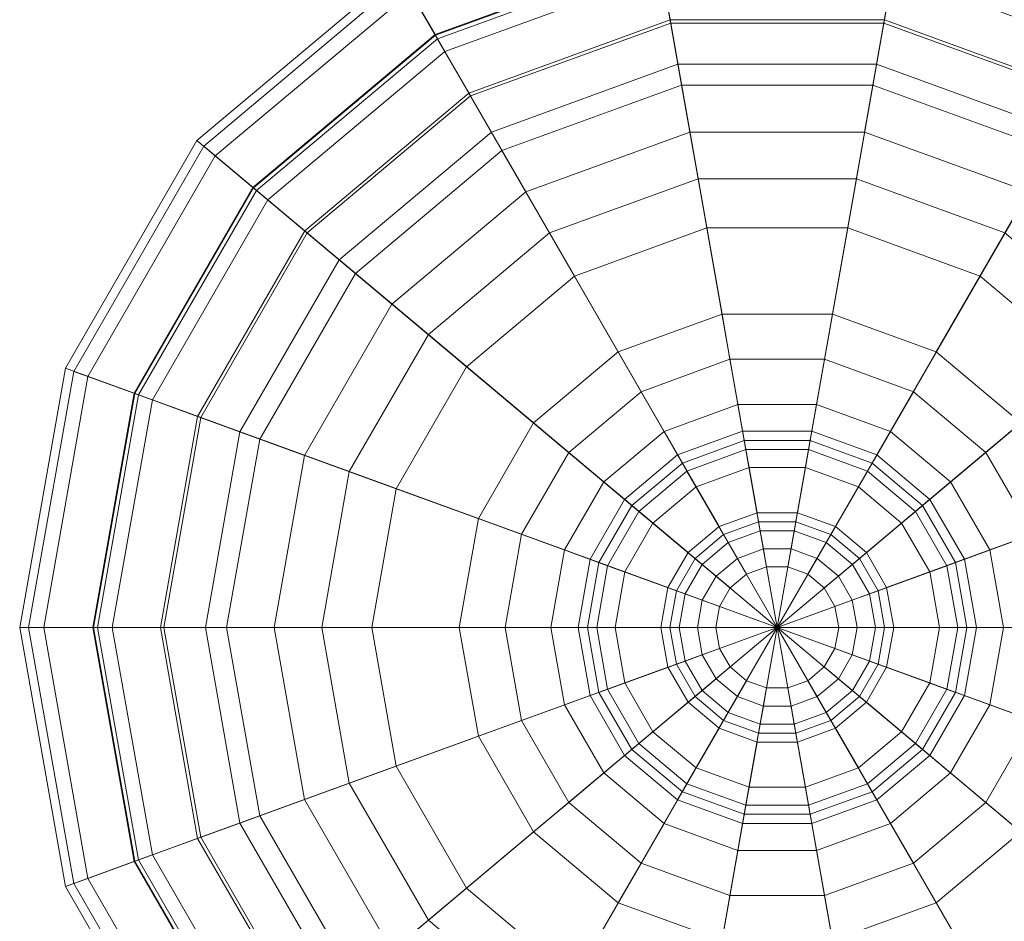
# Model space of a CAD drawing. Units: inches. Extents: x 375 to 1122, y 27 to 1069.
# Tile 120 of 155: x 717.909 to 719.669, y 890.59 to 892.201. Entities that reach past the tile are written whole.
import ezdxf

# ---------------------------------------------------------------- set-up
doc = ezdxf.new("R2010")
doc.units = ezdxf.units.IN
doc.layers.add('Furniture', color=30, linetype='Continuous', lineweight=18)

# ---------------------------------------------------------------- blocks, each defined once
blk = doc.blocks.new('A$C403C54AD')
for points in [[(1.180252, 0.891746, -0.031825), (1.180252, 0.857884, -0.028747), (1.180252, 0.857884, -0.028747), (1.16867, 0.889704, -0.031825)], [(1.191834, 0.889704, -0.031825), (1.180252, 0.857884, -0.028747), (1.180252, 0.857884, -0.028747), (1.180252, 0.891746, -0.031825)], [(1.16867, 0.889704, -0.031825), (1.180252, 0.857884, -0.028747), (1.180252, 0.857884, -0.028747), (1.158486, 0.883824, -0.031825)], [(1.202018, 0.883824, -0.031825), (1.180252, 0.857884, -0.028747), (1.180252, 0.857884, -0.028747), (1.191834, 0.889704, -0.031825)], [(1.158486, 0.883824, -0.031825), (1.180252, 0.857884, -0.028747), (1.180252, 0.857884, -0.028747), (1.150927, 0.874815, -0.031825)], [(1.209578, 0.874815, -0.031825), (1.180252, 0.857884, -0.028747), (1.180252, 0.857884, -0.028747), (1.202018, 0.883824, -0.031825)], [(1.171115, 0.868773, -0.02532), (1.160585, 0.881322, -0.028594), (1.153755, 0.873182, -0.028594), (1.167942, 0.864991, -0.02532)], [(1.192562, 0.864991, -0.02532), (1.206749, 0.873182, -0.028594), (1.199919, 0.881322, -0.028594), (1.189389, 0.868773, -0.02532)], [(1.180252, 0.878242, 0.061451), (1.180252, 0.868003, 0.054084), (1.176791, 0.867392, 0.054084), (1.173289, 0.877014, 0.061451)], [(1.187215, 0.877014, 0.061451), (1.183713, 0.867392, 0.054084), (1.180252, 0.868003, 0.054084), (1.180252, 0.878242, 0.061451)], [(1.1686, 0.87177, 0.063639), (1.164431, 0.876739, 0.073031), (1.158936, 0.87019, 0.073031), (1.164553, 0.866948, 0.063639)], [(1.173289, 0.877014, 0.061451), (1.176791, 0.867392, 0.054084), (1.173748, 0.865635, 0.054084), (1.167166, 0.873479, 0.061451)], [(1.193338, 0.873479, 0.061451), (1.186756, 0.865635, 0.054084), (1.183713, 0.867392, 0.054084), (1.187215, 0.877014, 0.061451)], [(1.195951, 0.866948, 0.063639), (1.201568, 0.87019, 0.073031), (1.196073, 0.876739, 0.073031), (1.191904, 0.87177, 0.063639)], [(1.180252, 0.866788, 0.057003), (1.180252, 0.876011, 0.063639), (1.174052, 0.874918, 0.063639), (1.177207, 0.866251, 0.057003)], [(1.183297, 0.866251, 0.057003), (1.186452, 0.874918, 0.063639), (1.180252, 0.876011, 0.063639), (1.180252, 0.866788, 0.057003)], [(1.153755, 0.873182, -0.028594), (1.150927, 0.874815, -0.031825), (1.146904, 0.863764, -0.031825), (1.15012, 0.863197, -0.028594)], [(1.150927, 0.874815, -0.031825), (1.180252, 0.857884, -0.028747), (1.180252, 0.857884, -0.028747), (1.146904, 0.863764, -0.031825)], [(1.15379, 0.873162, 0.131159), (1.151272, 0.874616, 0.117935), (1.147297, 0.863695, 0.117935), (1.15016, 0.86319, 0.131159)], [(1.177207, 0.866251, 0.057003), (1.174052, 0.874918, 0.063639), (1.1686, 0.87177, 0.063639), (1.174529, 0.864705, 0.057003)], [(1.2136, 0.863764, -0.031825), (1.180252, 0.857884, -0.028747), (1.180252, 0.857884, -0.028747), (1.209578, 0.874815, -0.031825)], [(1.185975, 0.864705, 0.057003), (1.191904, 0.87177, 0.063639), (1.186452, 0.874918, 0.063639), (1.183297, 0.866251, 0.057003)], [(1.151856, 0.874278, 0.089693), (1.156502, 0.871596, 0.071684), (1.153245, 0.862646, 0.071684), (1.147962, 0.863578, 0.089693)], [(1.167942, 0.864991, -0.02532), (1.153755, 0.873182, -0.028594), (1.15012, 0.863197, -0.028594), (1.166254, 0.860352, -0.02532)], [(1.167166, 0.873479, 0.061451), (1.173748, 0.865635, 0.054084), (1.171489, 0.862943, 0.054084), (1.162622, 0.868063, 0.061451)], [(1.197882, 0.868063, 0.061451), (1.189015, 0.862943, 0.054084), (1.186756, 0.865635, 0.054084), (1.193338, 0.873479, 0.061451)], [(1.19425, 0.860352, -0.02532), (1.210384, 0.863197, -0.028594), (1.206749, 0.873182, -0.028594), (1.192562, 0.864991, -0.02532)], [(1.158117, 0.870664, 0.140564), (1.15379, 0.873162, 0.131159), (1.15016, 0.86319, 0.131159), (1.155081, 0.862322, 0.140564)], [(1.153943, 0.873073, 0.117718), (1.156376, 0.871669, 0.130354), (1.153102, 0.862671, 0.130354), (1.150335, 0.863159, 0.117718)], [(1.154513, 0.872744, 0.090178), (1.153943, 0.873073, 0.117718), (1.150335, 0.863159, 0.117718), (1.150983, 0.863045, 0.090178)], [(1.158936, 0.87019, 0.073031), (1.154513, 0.872744, 0.090178), (1.150983, 0.863045, 0.090178), (1.156013, 0.862158, 0.073031)], [(1.156376, 0.871669, 0.130354), (1.160783, 0.869125, 0.140564), (1.158112, 0.861788, 0.140564), (1.153102, 0.862671, 0.130354)], [(1.156502, 0.871596, 0.071684), (1.162622, 0.868063, 0.061451), (1.160204, 0.861419, 0.061451), (1.153245, 0.862646, 0.071684)], [(1.174529, 0.864705, 0.057003), (1.1686, 0.87177, 0.063639), (1.164553, 0.866948, 0.063639), (1.172541, 0.862336, 0.057003)], [(1.187963, 0.862336, 0.057003), (1.195951, 0.866948, 0.063639), (1.191904, 0.87177, 0.063639), (1.185975, 0.864705, 0.057003)], [(1.176091, 0.869317, -0.022455), (1.17539, 0.871241, -0.02532), (1.171115, 0.868773, -0.02532), (1.172432, 0.867204, -0.022455)], [(1.188073, 0.867204, -0.022455), (1.189389, 0.868773, -0.02532), (1.185114, 0.871241, -0.02532), (1.184413, 0.869317, -0.022455)], [(1.160783, 0.869125, 0.140564), (1.158117, 0.870664, 0.140564), (1.155081, 0.862322, 0.140564), (1.158112, 0.861788, 0.140564)], [(1.164553, 0.866948, 0.063639), (1.158936, 0.87019, 0.073031), (1.156013, 0.862158, 0.073031), (1.1624, 0.861032, 0.063639)], [(1.180252, 0.865955, -0.020408), (1.180252, 0.87005, -0.022455), (1.176091, 0.869317, -0.022455), (1.177492, 0.865468, -0.020408)], [(1.183012, 0.865468, -0.020408), (1.184413, 0.869317, -0.022455), (1.180252, 0.87005, -0.022455), (1.180252, 0.865955, -0.020408)], [(1.177492, 0.865468, -0.020408), (1.176091, 0.869317, -0.022455), (1.172432, 0.867204, -0.022455), (1.175064, 0.864067, -0.020408)], [(1.18544, 0.864067, -0.020408), (1.188073, 0.867204, -0.022455), (1.184413, 0.869317, -0.022455), (1.183012, 0.865468, -0.020408)], [(1.172432, 0.867204, -0.022455), (1.171115, 0.868773, -0.02532), (1.167942, 0.864991, -0.02532), (1.169716, 0.863967, -0.022455)], [(1.190789, 0.863967, -0.022455), (1.192562, 0.864991, -0.02532), (1.189389, 0.868773, -0.02532), (1.188073, 0.867204, -0.022455)], [(1.162622, 0.868063, 0.061451), (1.171489, 0.862943, 0.054084), (1.170287, 0.859641, 0.054084), (1.160204, 0.861419, 0.061451)], [(1.180252, 0.868003, 0.054084), (1.180252, 0.863088, 0.053266), (1.178472, 0.862774, 0.053266), (1.176791, 0.867392, 0.054084)], [(1.183713, 0.867392, 0.054084), (1.182032, 0.862774, 0.053266), (1.180252, 0.863088, 0.053266), (1.180252, 0.868003, 0.054084)], [(1.2003, 0.861419, 0.061451), (1.190217, 0.859641, 0.054084), (1.189015, 0.862943, 0.054084), (1.197882, 0.868063, 0.061451)], [(1.175064, 0.864067, -0.020408), (1.172432, 0.867204, -0.022455), (1.169716, 0.863967, -0.022455), (1.173262, 0.861919, -0.020408)], [(1.176791, 0.867392, 0.054084), (1.178472, 0.862774, 0.053266), (1.176907, 0.861871, 0.053266), (1.173748, 0.865635, 0.054084)], [(1.186756, 0.865635, 0.054084), (1.183597, 0.861871, 0.053266), (1.182032, 0.862774, 0.053266), (1.183713, 0.867392, 0.054084)], [(1.187242, 0.861919, -0.020408), (1.190789, 0.863967, -0.022455), (1.188073, 0.867204, -0.022455), (1.18544, 0.864067, -0.020408)], [(1.172541, 0.862336, 0.057003), (1.164553, 0.866948, 0.063639), (1.1624, 0.861032, 0.063639), (1.171483, 0.85943, 0.057003)], [(1.180252, 0.857884, 0.055519), (1.180252, 0.866788, 0.057003), (1.177207, 0.866251, 0.057003), (1.180252, 0.857884, 0.055519)], [(1.180252, 0.857884, 0.055519), (1.183297, 0.866251, 0.057003), (1.180252, 0.866788, 0.057003), (1.180252, 0.857884, 0.055519)], [(1.189021, 0.85943, 0.057003), (1.198104, 0.861032, 0.063639), (1.195951, 0.866948, 0.063639), (1.187963, 0.862336, 0.057003)], [(1.180252, 0.857884, 0.055519), (1.177207, 0.866251, 0.057003), (1.174529, 0.864705, 0.057003), (1.180252, 0.857884, 0.055519)], [(1.180252, 0.866365, 0.0504), (1.180252, 0.862269, 0.048354), (1.178752, 0.862005, 0.048354), (1.177352, 0.865853, 0.0504)], [(1.180252, 0.865136, 0.052447), (1.180252, 0.866365, 0.0504), (1.177352, 0.865853, 0.0504), (1.177772, 0.864699, 0.052447)], [(1.183153, 0.865853, 0.0504), (1.181752, 0.862005, 0.048354), (1.180252, 0.862269, 0.048354), (1.180252, 0.866365, 0.0504)], [(1.182732, 0.864699, 0.052447), (1.183153, 0.865853, 0.0504), (1.180252, 0.866365, 0.0504), (1.180252, 0.865136, 0.052447)], [(1.180252, 0.857884, 0.055519), (1.185975, 0.864705, 0.057003), (1.183297, 0.866251, 0.057003), (1.180252, 0.857884, 0.055519)], [(1.177352, 0.865853, 0.0504), (1.178752, 0.862005, 0.048354), (1.177433, 0.861243, 0.048354), (1.174801, 0.86438, 0.0504)], [(1.177772, 0.864699, 0.052447), (1.177352, 0.865853, 0.0504), (1.174801, 0.86438, 0.0504), (1.175591, 0.863439, 0.052447)], [(1.180252, 0.862679, -0.015087), (1.180252, 0.865955, -0.020408), (1.177492, 0.865468, -0.020408), (1.178612, 0.862389, -0.015087)], [(1.181892, 0.862389, -0.015087), (1.183012, 0.865468, -0.020408), (1.180252, 0.865955, -0.020408), (1.180252, 0.862679, -0.015087)], [(1.185703, 0.86438, 0.0504), (1.183071, 0.861243, 0.048354), (1.181752, 0.862005, 0.048354), (1.183153, 0.865853, 0.0504)], [(1.184913, 0.863439, 0.052447), (1.185703, 0.86438, 0.0504), (1.183153, 0.865853, 0.0504), (1.182732, 0.864699, 0.052447)], [(1.173748, 0.865635, 0.054084), (1.176907, 0.861871, 0.053266), (1.175745, 0.860486, 0.053266), (1.171489, 0.862943, 0.054084)], [(1.178612, 0.862389, -0.015087), (1.177492, 0.865468, -0.020408), (1.175064, 0.864067, -0.020408), (1.17717, 0.861557, -0.015087)], [(1.183334, 0.861557, -0.015087), (1.18544, 0.864067, -0.020408), (1.183012, 0.865468, -0.020408), (1.181892, 0.862389, -0.015087)], [(1.189015, 0.862943, 0.054084), (1.184759, 0.860486, 0.053266), (1.183597, 0.861871, 0.053266), (1.186756, 0.865635, 0.054084)], [(1.169716, 0.863967, -0.022455), (1.167942, 0.864991, -0.02532), (1.166254, 0.860352, -0.02532), (1.16827, 0.859997, -0.022455)], [(1.180252, 0.863088, 0.053266), (1.180252, 0.865136, 0.052447), (1.177772, 0.864699, 0.052447), (1.178472, 0.862774, 0.053266)], [(1.182032, 0.862774, 0.053266), (1.182732, 0.864699, 0.052447), (1.180252, 0.865136, 0.052447), (1.180252, 0.863088, 0.053266)], [(1.192234, 0.859997, -0.022455), (1.19425, 0.860352, -0.02532), (1.192562, 0.864991, -0.02532), (1.190789, 0.863967, -0.022455)], [(1.180252, 0.857884, 0.055519), (1.174529, 0.864705, 0.057003), (1.172541, 0.862336, 0.057003), (1.180252, 0.857884, 0.055519)], [(1.174801, 0.86438, 0.0504), (1.177433, 0.861243, 0.048354), (1.176454, 0.860076, 0.048354), (1.172908, 0.862124, 0.0504)], [(1.175591, 0.863439, 0.052447), (1.174801, 0.86438, 0.0504), (1.172908, 0.862124, 0.0504), (1.173972, 0.86151, 0.052447)], [(1.178472, 0.862774, 0.053266), (1.177772, 0.864699, 0.052447), (1.175591, 0.863439, 0.052447), (1.176907, 0.861871, 0.053266)], [(1.180252, 0.857884, 0.055519), (1.187963, 0.862336, 0.057003), (1.185975, 0.864705, 0.057003), (1.180252, 0.857884, 0.055519)], [(1.183597, 0.861871, 0.053266), (1.184913, 0.863439, 0.052447), (1.182732, 0.864699, 0.052447), (1.182032, 0.862774, 0.053266)], [(1.187596, 0.862124, 0.0504), (1.18405, 0.860076, 0.048354), (1.183071, 0.861243, 0.048354), (1.185703, 0.86438, 0.0504)], [(1.186532, 0.86151, 0.052447), (1.187596, 0.862124, 0.0504), (1.185703, 0.86438, 0.0504), (1.184913, 0.863439, 0.052447)], [(1.173262, 0.861919, -0.020408), (1.169716, 0.863967, -0.022455), (1.16827, 0.859997, -0.022455), (1.172304, 0.859285, -0.020408)], [(1.17717, 0.861557, -0.015087), (1.175064, 0.864067, -0.020408), (1.173262, 0.861919, -0.020408), (1.1761, 0.860281, -0.015087)], [(1.184404, 0.860281, -0.015087), (1.187242, 0.861919, -0.020408), (1.18544, 0.864067, -0.020408), (1.183334, 0.861557, -0.015087)], [(1.1882, 0.859285, -0.020408), (1.192234, 0.859997, -0.022455), (1.190789, 0.863967, -0.022455), (1.187242, 0.861919, -0.020408)], [(1.146904, 0.863764, -0.031825), (1.180252, 0.857884, -0.028747), (1.180252, 0.857884, -0.028747), (1.146904, 0.852004, -0.031825)], [(1.147962, 0.863578, 0.089693), (1.153245, 0.862646, 0.071684), (1.153245, 0.853122, 0.071684), (1.147962, 0.85219, 0.089693)], [(1.2136, 0.852004, -0.031825), (1.180252, 0.857884, -0.028747), (1.180252, 0.857884, -0.028747), (1.2136, 0.863764, -0.031825)], [(1.166254, 0.860352, -0.02532), (1.15012, 0.863197, -0.028594), (1.15012, 0.852571, -0.028594), (1.166254, 0.855416, -0.02532)], [(1.155081, 0.862322, 0.140564), (1.15016, 0.86319, 0.131159), (1.15016, 0.852578, 0.131159), (1.155081, 0.853446, 0.140564)], [(1.150335, 0.863159, 0.117718), (1.153102, 0.862671, 0.130354), (1.153102, 0.853097, 0.130354), (1.150335, 0.852609, 0.117718)], [(1.176907, 0.861871, 0.053266), (1.175591, 0.863439, 0.052447), (1.173972, 0.86151, 0.052447), (1.175745, 0.860486, 0.053266)], [(1.184759, 0.860486, 0.053266), (1.186532, 0.86151, 0.052447), (1.184913, 0.863439, 0.052447), (1.183597, 0.861871, 0.053266)], [(1.156013, 0.862158, 0.073031), (1.150983, 0.863045, 0.090178), (1.150983, 0.852723, 0.090178), (1.156013, 0.85361, 0.073031)], [(1.153102, 0.862671, 0.130354), (1.158112, 0.861788, 0.140564), (1.158112, 0.85398, 0.140564), (1.153102, 0.853097, 0.130354)], [(1.153245, 0.862646, 0.071684), (1.160204, 0.861419, 0.061451), (1.160204, 0.854349, 0.061451), (1.153245, 0.853122, 0.071684)], [(1.171489, 0.862943, 0.054084), (1.175745, 0.860486, 0.053266), (1.175127, 0.858788, 0.053266), (1.170287, 0.859641, 0.054084)], [(1.180252, 0.86145, -0.006492), (1.180252, 0.862679, -0.015087), (1.178612, 0.862389, -0.015087), (1.179032, 0.861235, -0.006492)], [(1.181472, 0.861235, -0.006492), (1.181892, 0.862389, -0.015087), (1.180252, 0.862679, -0.015087), (1.180252, 0.86145, -0.006492)], [(1.190217, 0.859641, 0.054084), (1.185377, 0.858788, 0.053266), (1.184759, 0.860486, 0.053266), (1.189015, 0.862943, 0.054084)], [(1.158112, 0.861788, 0.140564), (1.155081, 0.862322, 0.140564), (1.155081, 0.853446, 0.140564), (1.158112, 0.85398, 0.140564)], [(1.180252, 0.857884, 0.055519), (1.172541, 0.862336, 0.057003), (1.171483, 0.85943, 0.057003), (1.180252, 0.857884, 0.055519)], [(1.179032, 0.861235, -0.006492), (1.178612, 0.862389, -0.015087), (1.17717, 0.861557, -0.015087), (1.17796, 0.860616, -0.006492)], [(1.180252, 0.862269, 0.048354), (1.180252, 0.860631, 0.041805), (1.179313, 0.860465, 0.041805), (1.178752, 0.862005, 0.048354)], [(1.180252, 0.857884, 0.055519), (1.189021, 0.85943, 0.057003), (1.187963, 0.862336, 0.057003), (1.180252, 0.857884, 0.055519)], [(1.181752, 0.862005, 0.048354), (1.181191, 0.860465, 0.041805), (1.180252, 0.860631, 0.041805), (1.180252, 0.862269, 0.048354)], [(1.182544, 0.860616, -0.006492), (1.183334, 0.861557, -0.015087), (1.181892, 0.862389, -0.015087), (1.181472, 0.861235, -0.006492)], [(1.1624, 0.861032, 0.063639), (1.156013, 0.862158, 0.073031), (1.156013, 0.85361, 0.073031), (1.1624, 0.854736, 0.063639)], [(1.173972, 0.86151, 0.052447), (1.172908, 0.862124, 0.0504), (1.1719, 0.859357, 0.0504), (1.17311, 0.859143, 0.052447)], [(1.172908, 0.862124, 0.0504), (1.176454, 0.860076, 0.048354), (1.175934, 0.858645, 0.048354), (1.1719, 0.859357, 0.0504)], [(1.1761, 0.860281, -0.015087), (1.173262, 0.861919, -0.020408), (1.172304, 0.859285, -0.020408), (1.17553, 0.858717, -0.015087)], [(1.178752, 0.862005, 0.048354), (1.179313, 0.860465, 0.041805), (1.178486, 0.859988, 0.041805), (1.177433, 0.861243, 0.048354)], [(1.183071, 0.861243, 0.048354), (1.182018, 0.859988, 0.041805), (1.181191, 0.860465, 0.041805), (1.181752, 0.862005, 0.048354)], [(1.188604, 0.859357, 0.0504), (1.18457, 0.858645, 0.048354), (1.18405, 0.860076, 0.048354), (1.187596, 0.862124, 0.0504)], [(1.184974, 0.858717, -0.015087), (1.1882, 0.859285, -0.020408), (1.187242, 0.861919, -0.020408), (1.184404, 0.860281, -0.015087)], [(1.187394, 0.859143, 0.052447), (1.188604, 0.859357, 0.0504), (1.187596, 0.862124, 0.0504), (1.186532, 0.86151, 0.052447)], [(1.160204, 0.861419, 0.061451), (1.170287, 0.859641, 0.054084), (1.170287, 0.856127, 0.054084), (1.160204, 0.854349, 0.061451)], [(1.175745, 0.860486, 0.053266), (1.173972, 0.86151, 0.052447), (1.17311, 0.859143, 0.052447), (1.175127, 0.858788, 0.053266)], [(1.17796, 0.860616, -0.006492), (1.17717, 0.861557, -0.015087), (1.1761, 0.860281, -0.015087), (1.177164, 0.859667, -0.006492)], [(1.180252, 0.860631, 0.041805), (1.180252, 0.86145, -0.006492), (1.179032, 0.861235, -0.006492), (1.179313, 0.860465, 0.041805)], [(1.181191, 0.860465, 0.041805), (1.181472, 0.861235, -0.006492), (1.180252, 0.86145, -0.006492), (1.180252, 0.860631, 0.041805)], [(1.18334, 0.859667, -0.006492), (1.184404, 0.860281, -0.015087), (1.183334, 0.861557, -0.015087), (1.182544, 0.860616, -0.006492)], [(1.185377, 0.858788, 0.053266), (1.187394, 0.859143, 0.052447), (1.186532, 0.86151, 0.052447), (1.184759, 0.860486, 0.053266)], [(1.2003, 0.854349, 0.061451), (1.190217, 0.856127, 0.054084), (1.190217, 0.859641, 0.054084), (1.2003, 0.861419, 0.061451)], [(1.171483, 0.85943, 0.057003), (1.1624, 0.861032, 0.063639), (1.1624, 0.854736, 0.063639), (1.171483, 0.856338, 0.057003)], [(1.177433, 0.861243, 0.048354), (1.178486, 0.859988, 0.041805), (1.177873, 0.859257, 0.041805), (1.176454, 0.860076, 0.048354)], [(1.179313, 0.860465, 0.041805), (1.179032, 0.861235, -0.006492), (1.17796, 0.860616, -0.006492), (1.178486, 0.859988, 0.041805)], [(1.182018, 0.859988, 0.041805), (1.182544, 0.860616, -0.006492), (1.181472, 0.861235, -0.006492), (1.181191, 0.860465, 0.041805)], [(1.18405, 0.860076, 0.048354), (1.182631, 0.859257, 0.041805), (1.182018, 0.859988, 0.041805), (1.183071, 0.861243, 0.048354)], [(1.189021, 0.856338, 0.057003), (1.198104, 0.854736, 0.063639), (1.198104, 0.861032, 0.063639), (1.189021, 0.85943, 0.057003)], [(1.178486, 0.859988, 0.041805), (1.17796, 0.860616, -0.006492), (1.177164, 0.859667, -0.006492), (1.177873, 0.859257, 0.041805)], [(1.182631, 0.859257, 0.041805), (1.18334, 0.859667, -0.006492), (1.182544, 0.860616, -0.006492), (1.182018, 0.859988, 0.041805)], [(1.16827, 0.859997, -0.022455), (1.166254, 0.860352, -0.02532), (1.166254, 0.855416, -0.02532), (1.16827, 0.855771, -0.022455)], [(1.172304, 0.859285, -0.020408), (1.16827, 0.859997, -0.022455), (1.16827, 0.855771, -0.022455), (1.172304, 0.856482, -0.020408)], [(1.177164, 0.859667, -0.006492), (1.1761, 0.860281, -0.015087), (1.17553, 0.858717, -0.015087), (1.17674, 0.858503, -0.006492)], [(1.176454, 0.860076, 0.048354), (1.177873, 0.859257, 0.041805), (1.177547, 0.858361, 0.041805), (1.175934, 0.858645, 0.048354)], [(1.18457, 0.858645, 0.048354), (1.182957, 0.858361, 0.041805), (1.182631, 0.859257, 0.041805), (1.18405, 0.860076, 0.048354)], [(1.183764, 0.858503, -0.006492), (1.184974, 0.858717, -0.015087), (1.184404, 0.860281, -0.015087), (1.18334, 0.859667, -0.006492)], [(1.1882, 0.856482, -0.020408), (1.192234, 0.855771, -0.022455), (1.192234, 0.859997, -0.022455), (1.1882, 0.859285, -0.020408)], [(1.192234, 0.855771, -0.022455), (1.19425, 0.855416, -0.02532), (1.19425, 0.860352, -0.02532), (1.192234, 0.859997, -0.022455)], [(1.170287, 0.859641, 0.054084), (1.175127, 0.858788, 0.053266), (1.175127, 0.85698, 0.053266), (1.170287, 0.856127, 0.054084)], [(1.177873, 0.859257, 0.041805), (1.177164, 0.859667, -0.006492), (1.17674, 0.858503, -0.006492), (1.177547, 0.858361, 0.041805)], [(1.182957, 0.858361, 0.041805), (1.183764, 0.858503, -0.006492), (1.18334, 0.859667, -0.006492), (1.182631, 0.859257, 0.041805)], [(1.190217, 0.856127, 0.054084), (1.185377, 0.85698, 0.053266), (1.185377, 0.858788, 0.053266), (1.190217, 0.859641, 0.054084)], [(1.180252, 0.857884, 0.055519), (1.171483, 0.85943, 0.057003), (1.171483, 0.856338, 0.057003), (1.180252, 0.857884, 0.055519)], [(1.17311, 0.859143, 0.052447), (1.1719, 0.859357, 0.0504), (1.1719, 0.856411, 0.0504), (1.17311, 0.856625, 0.052447)], [(1.1719, 0.859357, 0.0504), (1.175934, 0.858645, 0.048354), (1.175934, 0.857123, 0.048354), (1.1719, 0.856411, 0.0504)], [(1.17553, 0.858717, -0.015087), (1.172304, 0.859285, -0.020408), (1.172304, 0.856482, -0.020408), (1.17553, 0.857051, -0.015087)], [(1.175127, 0.858788, 0.053266), (1.17311, 0.859143, 0.052447), (1.17311, 0.856625, 0.052447), (1.175127, 0.85698, 0.053266)], [(1.180252, 0.857884, 0.055519), (1.189021, 0.856338, 0.057003), (1.189021, 0.85943, 0.057003), (1.180252, 0.857884, 0.055519)], [(1.188604, 0.856411, 0.0504), (1.18457, 0.857123, 0.048354), (1.18457, 0.858645, 0.048354), (1.188604, 0.859357, 0.0504)], [(1.184974, 0.857051, -0.015087), (1.1882, 0.856482, -0.020408), (1.1882, 0.859285, -0.020408), (1.184974, 0.858717, -0.015087)], [(1.185377, 0.85698, 0.053266), (1.187394, 0.856625, 0.052447), (1.187394, 0.859143, 0.052447), (1.185377, 0.858788, 0.053266)], [(1.187394, 0.856625, 0.052447), (1.188604, 0.856411, 0.0504), (1.188604, 0.859357, 0.0504), (1.187394, 0.859143, 0.052447)], [(1.17674, 0.858503, -0.006492), (1.17553, 0.858717, -0.015087), (1.17553, 0.857051, -0.015087), (1.17674, 0.857265, -0.006492)], [(1.183764, 0.857265, -0.006492), (1.184974, 0.857051, -0.015087), (1.184974, 0.858717, -0.015087), (1.183764, 0.858503, -0.006492)], [(1.175934, 0.858645, 0.048354), (1.177547, 0.858361, 0.041805), (1.177547, 0.857407, 0.041805), (1.175934, 0.857123, 0.048354)], [(1.177547, 0.858361, 0.041805), (1.17674, 0.858503, -0.006492), (1.17674, 0.857265, -0.006492), (1.177547, 0.857407, 0.041805)], [(1.18457, 0.857123, 0.048354), (1.182957, 0.857407, 0.041805), (1.182957, 0.858361, 0.041805), (1.18457, 0.858645, 0.048354)], [(1.182957, 0.857407, 0.041805), (1.183764, 0.857265, -0.006492), (1.183764, 0.858503, -0.006492), (1.182957, 0.858361, 0.041805)], [(1.146904, 0.852004, -0.031825), (1.180252, 0.857884, -0.028747), (1.180252, 0.857884, -0.028747), (1.150927, 0.840953, -0.031825)], [(1.150927, 0.840953, -0.031825), (1.180252, 0.857884, -0.028747), (1.180252, 0.857884, -0.028747), (1.158486, 0.831944, -0.031825)], [(1.158486, 0.831944, -0.031825), (1.180252, 0.857884, -0.028747), (1.180252, 0.857884, -0.028747), (1.16867, 0.826064, -0.031825)], [(1.16867, 0.826064, -0.031825), (1.180252, 0.857884, -0.028747), (1.180252, 0.857884, -0.028747), (1.180252, 0.824022, -0.031825)], [(1.180252, 0.857884, 0.055519), (1.171483, 0.856338, 0.057003), (1.172541, 0.853432, 0.057003), (1.180252, 0.857884, 0.055519)], [(1.180252, 0.857884, 0.055519), (1.172541, 0.853432, 0.057003), (1.174529, 0.851063, 0.057003), (1.180252, 0.857884, 0.055519)], [(1.180252, 0.857884, 0.055519), (1.174529, 0.851063, 0.057003), (1.177207, 0.849517, 0.057003), (1.180252, 0.857884, 0.055519)], [(1.180252, 0.857884, 0.055519), (1.177207, 0.849517, 0.057003), (1.180252, 0.84898, 0.057003), (1.180252, 0.857884, 0.055519)], [(1.180252, 0.857884, 0.055519), (1.187963, 0.853432, 0.057003), (1.189021, 0.856338, 0.057003), (1.180252, 0.857884, 0.055519)], [(1.180252, 0.857884, 0.055519), (1.185975, 0.851063, 0.057003), (1.187963, 0.853432, 0.057003), (1.180252, 0.857884, 0.055519)], [(1.180252, 0.857884, 0.055519), (1.183297, 0.849517, 0.057003), (1.185975, 0.851063, 0.057003), (1.180252, 0.857884, 0.055519)], [(1.180252, 0.857884, 0.055519), (1.180252, 0.84898, 0.057003), (1.183297, 0.849517, 0.057003), (1.180252, 0.857884, 0.055519)], [(1.209578, 0.840953, -0.031825), (1.180252, 0.857884, -0.028747), (1.180252, 0.857884, -0.028747), (1.2136, 0.852004, -0.031825)], [(1.202018, 0.831944, -0.031825), (1.180252, 0.857884, -0.028747), (1.180252, 0.857884, -0.028747), (1.209578, 0.840953, -0.031825)], [(1.191834, 0.826064, -0.031825), (1.180252, 0.857884, -0.028747), (1.180252, 0.857884, -0.028747), (1.202018, 0.831944, -0.031825)], [(1.180252, 0.824022, -0.031825), (1.180252, 0.857884, -0.028747), (1.180252, 0.857884, -0.028747), (1.191834, 0.826064, -0.031825)], [(1.175934, 0.857123, 0.048354), (1.177547, 0.857407, 0.041805), (1.177873, 0.856511, 0.041805), (1.176454, 0.855691, 0.048354)], [(1.177547, 0.857407, 0.041805), (1.17674, 0.857265, -0.006492), (1.177164, 0.856101, -0.006492), (1.177873, 0.856511, 0.041805)], [(1.18405, 0.855691, 0.048354), (1.182631, 0.856511, 0.041805), (1.182957, 0.857407, 0.041805), (1.18457, 0.857123, 0.048354)], [(1.182631, 0.856511, 0.041805), (1.18334, 0.856101, -0.006492), (1.183764, 0.857265, -0.006492), (1.182957, 0.857407, 0.041805)], [(1.170287, 0.856127, 0.054084), (1.175127, 0.85698, 0.053266), (1.175745, 0.855282, 0.053266), (1.171489, 0.852825, 0.054084)], [(1.1719, 0.856411, 0.0504), (1.175934, 0.857123, 0.048354), (1.176454, 0.855691, 0.048354), (1.172908, 0.853644, 0.0504)], [(1.17553, 0.857051, -0.015087), (1.172304, 0.856482, -0.020408), (1.173262, 0.853848, -0.020408), (1.1761, 0.855487, -0.015087)], [(1.175127, 0.85698, 0.053266), (1.17311, 0.856625, 0.052447), (1.173972, 0.854258, 0.052447), (1.175745, 0.855282, 0.053266)], [(1.17674, 0.857265, -0.006492), (1.17553, 0.857051, -0.015087), (1.1761, 0.855487, -0.015087), (1.177164, 0.856101, -0.006492)], [(1.18334, 0.856101, -0.006492), (1.184404, 0.855487, -0.015087), (1.184974, 0.857051, -0.015087), (1.183764, 0.857265, -0.006492)], [(1.187596, 0.853644, 0.0504), (1.18405, 0.855691, 0.048354), (1.18457, 0.857123, 0.048354), (1.188604, 0.856411, 0.0504)], [(1.184404, 0.855487, -0.015087), (1.187242, 0.853848, -0.020408), (1.1882, 0.856482, -0.020408), (1.184974, 0.857051, -0.015087)], [(1.184759, 0.855282, 0.053266), (1.186532, 0.854258, 0.052447), (1.187394, 0.856625, 0.052447), (1.185377, 0.85698, 0.053266)], [(1.189015, 0.852825, 0.054084), (1.184759, 0.855282, 0.053266), (1.185377, 0.85698, 0.053266), (1.190217, 0.856127, 0.054084)], [(1.172304, 0.856482, -0.020408), (1.16827, 0.855771, -0.022455), (1.169716, 0.851801, -0.022455), (1.173262, 0.853848, -0.020408)], [(1.17311, 0.856625, 0.052447), (1.1719, 0.856411, 0.0504), (1.172908, 0.853644, 0.0504), (1.173972, 0.854258, 0.052447)], [(1.176454, 0.855691, 0.048354), (1.177873, 0.856511, 0.041805), (1.178486, 0.85578, 0.041805), (1.177433, 0.854525, 0.048354)], [(1.177873, 0.856511, 0.041805), (1.177164, 0.856101, -0.006492), (1.17796, 0.855152, -0.006492), (1.178486, 0.85578, 0.041805)], [(1.183071, 0.854525, 0.048354), (1.182018, 0.85578, 0.041805), (1.182631, 0.856511, 0.041805), (1.18405, 0.855691, 0.048354)], [(1.182018, 0.85578, 0.041805), (1.182544, 0.855152, -0.006492), (1.18334, 0.856101, -0.006492), (1.182631, 0.856511, 0.041805)], [(1.186532, 0.854258, 0.052447), (1.187596, 0.853644, 0.0504), (1.188604, 0.856411, 0.0504), (1.187394, 0.856625, 0.052447)], [(1.187242, 0.853848, -0.020408), (1.190789, 0.851801, -0.022455), (1.192234, 0.855771, -0.022455), (1.1882, 0.856482, -0.020408)], [(1.160204, 0.854349, 0.061451), (1.170287, 0.856127, 0.054084), (1.171489, 0.852825, 0.054084), (1.162622, 0.847705, 0.061451)], [(1.171483, 0.856338, 0.057003), (1.1624, 0.854736, 0.063639), (1.164553, 0.84882, 0.063639), (1.172541, 0.853432, 0.057003)], [(1.177164, 0.856101, -0.006492), (1.1761, 0.855487, -0.015087), (1.17717, 0.854211, -0.015087), (1.17796, 0.855152, -0.006492)], [(1.182544, 0.855152, -0.006492), (1.183334, 0.854211, -0.015087), (1.184404, 0.855487, -0.015087), (1.18334, 0.856101, -0.006492)], [(1.187963, 0.853432, 0.057003), (1.195951, 0.84882, 0.063639), (1.198104, 0.854736, 0.063639), (1.189021, 0.856338, 0.057003)], [(1.197882, 0.847705, 0.061451), (1.189015, 0.852825, 0.054084), (1.190217, 0.856127, 0.054084), (1.2003, 0.854349, 0.061451)], [(1.16827, 0.855771, -0.022455), (1.166254, 0.855416, -0.02532), (1.167942, 0.850777, -0.02532), (1.169716, 0.851801, -0.022455)], [(1.172908, 0.853644, 0.0504), (1.176454, 0.855691, 0.048354), (1.177433, 0.854525, 0.048354), (1.174801, 0.851387, 0.0504)], [(1.177433, 0.854525, 0.048354), (1.178486, 0.85578, 0.041805), (1.179313, 0.855303, 0.041805), (1.178752, 0.853763, 0.048354)], [(1.178486, 0.85578, 0.041805), (1.17796, 0.855152, -0.006492), (1.179032, 0.854533, -0.006492), (1.179313, 0.855303, 0.041805)], [(1.181752, 0.853763, 0.048354), (1.181191, 0.855303, 0.041805), (1.182018, 0.85578, 0.041805), (1.183071, 0.854525, 0.048354)], [(1.181191, 0.855303, 0.041805), (1.181472, 0.854533, -0.006492), (1.182544, 0.855152, -0.006492), (1.182018, 0.85578, 0.041805)], [(1.185703, 0.851387, 0.0504), (1.183071, 0.854525, 0.048354), (1.18405, 0.855691, 0.048354), (1.187596, 0.853644, 0.0504)], [(1.190789, 0.851801, -0.022455), (1.192562, 0.850777, -0.02532), (1.19425, 0.855416, -0.02532), (1.192234, 0.855771, -0.022455)], [(1.166254, 0.855416, -0.02532), (1.15012, 0.852571, -0.028594), (1.153755, 0.842586, -0.028594), (1.167942, 0.850777, -0.02532)], [(1.171489, 0.852825, 0.054084), (1.175745, 0.855282, 0.053266), (1.176907, 0.853897, 0.053266), (1.173748, 0.850133, 0.054084)], [(1.1761, 0.855487, -0.015087), (1.173262, 0.853848, -0.020408), (1.175064, 0.851701, -0.020408), (1.17717, 0.854211, -0.015087)], [(1.175745, 0.855282, 0.053266), (1.173972, 0.854258, 0.052447), (1.175591, 0.852329, 0.052447), (1.176907, 0.853897, 0.053266)], [(1.17796, 0.855152, -0.006492), (1.17717, 0.854211, -0.015087), (1.178612, 0.853379, -0.015087), (1.179032, 0.854533, -0.006492)], [(1.178752, 0.853763, 0.048354), (1.179313, 0.855303, 0.041805), (1.180252, 0.855137, 0.041805), (1.180252, 0.853499, 0.048354)], [(1.179313, 0.855303, 0.041805), (1.179032, 0.854533, -0.006492), (1.180252, 0.854318, -0.006492), (1.180252, 0.855137, 0.041805)], [(1.180252, 0.853499, 0.048354), (1.180252, 0.855137, 0.041805), (1.181191, 0.855303, 0.041805), (1.181752, 0.853763, 0.048354)], [(1.180252, 0.855137, 0.041805), (1.180252, 0.854318, -0.006492), (1.181472, 0.854533, -0.006492), (1.181191, 0.855303, 0.041805)], [(1.181472, 0.854533, -0.006492), (1.181892, 0.853379, -0.015087), (1.183334, 0.854211, -0.015087), (1.182544, 0.855152, -0.006492)], [(1.183334, 0.854211, -0.015087), (1.18544, 0.851701, -0.020408), (1.187242, 0.853848, -0.020408), (1.184404, 0.855487, -0.015087)], [(1.183597, 0.853897, 0.053266), (1.184913, 0.852329, 0.052447), (1.186532, 0.854258, 0.052447), (1.184759, 0.855282, 0.053266)], [(1.186756, 0.850133, 0.054084), (1.183597, 0.853897, 0.053266), (1.184759, 0.855282, 0.053266), (1.189015, 0.852825, 0.054084)], [(1.192562, 0.850777, -0.02532), (1.206749, 0.842586, -0.028594), (1.210384, 0.852571, -0.028594), (1.19425, 0.855416, -0.02532)], [(1.1624, 0.854736, 0.063639), (1.156013, 0.85361, 0.073031), (1.158936, 0.845577, 0.073031), (1.164553, 0.84882, 0.063639)], [(1.153245, 0.853122, 0.071684), (1.160204, 0.854349, 0.061451), (1.162622, 0.847705, 0.061451), (1.156502, 0.844172, 0.071684)], [(1.173972, 0.854258, 0.052447), (1.172908, 0.853644, 0.0504), (1.174801, 0.851387, 0.0504), (1.175591, 0.852329, 0.052447)], [(1.174801, 0.851387, 0.0504), (1.177433, 0.854525, 0.048354), (1.178752, 0.853763, 0.048354), (1.177352, 0.849915, 0.0504)], [(1.179032, 0.854533, -0.006492), (1.178612, 0.853379, -0.015087), (1.180252, 0.853089, -0.015087), (1.180252, 0.854318, -0.006492)], [(1.180252, 0.854318, -0.006492), (1.180252, 0.853089, -0.015087), (1.181892, 0.853379, -0.015087), (1.181472, 0.854533, -0.006492)], [(1.183153, 0.849915, 0.0504), (1.181752, 0.853763, 0.048354), (1.183071, 0.854525, 0.048354), (1.185703, 0.851387, 0.0504)], [(1.184913, 0.852329, 0.052447), (1.185703, 0.851387, 0.0504), (1.187596, 0.853644, 0.0504), (1.186532, 0.854258, 0.052447)], [(1.153102, 0.853097, 0.130354), (1.158112, 0.85398, 0.140564), (1.160783, 0.846643, 0.140564), (1.156376, 0.844099, 0.130354)], [(1.158112, 0.85398, 0.140564), (1.155081, 0.853446, 0.140564), (1.158117, 0.845104, 0.140564), (1.160783, 0.846643, 0.140564)], [(1.173262, 0.853848, -0.020408), (1.169716, 0.851801, -0.022455), (1.172432, 0.848564, -0.022455), (1.175064, 0.851701, -0.020408)], [(1.173748, 0.850133, 0.054084), (1.176907, 0.853897, 0.053266), (1.178472, 0.852994, 0.053266), (1.176791, 0.848375, 0.054084)], [(1.17717, 0.854211, -0.015087), (1.175064, 0.851701, -0.020408), (1.177492, 0.8503, -0.020408), (1.178612, 0.853379, -0.015087)], [(1.176907, 0.853897, 0.053266), (1.175591, 0.852329, 0.052447), (1.177772, 0.851069, 0.052447), (1.178472, 0.852994, 0.053266)], [(1.181892, 0.853379, -0.015087), (1.183012, 0.8503, -0.020408), (1.18544, 0.851701, -0.020408), (1.183334, 0.854211, -0.015087)], [(1.182032, 0.852994, 0.053266), (1.182732, 0.851069, 0.052447), (1.184913, 0.852329, 0.052447), (1.183597, 0.853897, 0.053266)], [(1.183713, 0.848375, 0.054084), (1.182032, 0.852994, 0.053266), (1.183597, 0.853897, 0.053266), (1.186756, 0.850133, 0.054084)], [(1.18544, 0.851701, -0.020408), (1.188073, 0.848564, -0.022455), (1.190789, 0.851801, -0.022455), (1.187242, 0.853848, -0.020408)], [(1.155081, 0.853446, 0.140564), (1.15016, 0.852578, 0.131159), (1.15379, 0.842606, 0.131159), (1.158117, 0.845104, 0.140564)], [(1.156013, 0.85361, 0.073031), (1.150983, 0.852723, 0.090178), (1.154513, 0.843024, 0.090178), (1.158936, 0.845577, 0.073031)], [(1.172541, 0.853432, 0.057003), (1.164553, 0.84882, 0.063639), (1.1686, 0.843998, 0.063639), (1.174529, 0.851063, 0.057003)], [(1.177352, 0.849915, 0.0504), (1.178752, 0.853763, 0.048354), (1.180252, 0.853499, 0.048354), (1.180252, 0.849403, 0.0504)], [(1.178612, 0.853379, -0.015087), (1.177492, 0.8503, -0.020408), (1.180252, 0.849813, -0.020408), (1.180252, 0.853089, -0.015087)], [(1.180252, 0.849403, 0.0504), (1.180252, 0.853499, 0.048354), (1.181752, 0.853763, 0.048354), (1.183153, 0.849915, 0.0504)], [(1.180252, 0.853089, -0.015087), (1.180252, 0.849813, -0.020408), (1.183012, 0.8503, -0.020408), (1.181892, 0.853379, -0.015087)], [(1.185975, 0.851063, 0.057003), (1.191904, 0.843998, 0.063639), (1.195951, 0.84882, 0.063639), (1.187963, 0.853432, 0.057003)], [(1.147962, 0.85219, 0.089693), (1.153245, 0.853122, 0.071684), (1.156502, 0.844172, 0.071684), (1.151856, 0.84149, 0.089693)], [(1.150335, 0.852609, 0.117718), (1.153102, 0.853097, 0.130354), (1.156376, 0.844099, 0.130354), (1.153943, 0.842695, 0.117718)], [(1.176791, 0.848375, 0.054084), (1.178472, 0.852994, 0.053266), (1.180252, 0.85268, 0.053266), (1.180252, 0.847765, 0.054084)], [(1.178472, 0.852994, 0.053266), (1.177772, 0.851069, 0.052447), (1.180252, 0.850632, 0.052447), (1.180252, 0.85268, 0.053266)], [(1.180252, 0.85268, 0.053266), (1.180252, 0.850632, 0.052447), (1.182732, 0.851069, 0.052447), (1.182032, 0.852994, 0.053266)], [(1.180252, 0.847765, 0.054084), (1.180252, 0.85268, 0.053266), (1.182032, 0.852994, 0.053266), (1.183713, 0.848375, 0.054084)], [(1.15012, 0.852571, -0.028594), (1.146904, 0.852004, -0.031825), (1.150927, 0.840953, -0.031825), (1.153755, 0.842586, -0.028594)], [(1.15016, 0.852578, 0.131159), (1.147297, 0.852073, 0.117935), (1.151272, 0.841152, 0.117935), (1.15379, 0.842606, 0.131159)], [(1.150983, 0.852723, 0.090178), (1.150335, 0.852609, 0.117718), (1.153943, 0.842695, 0.117718), (1.154513, 0.843024, 0.090178)], [(1.162622, 0.847705, 0.061451), (1.171489, 0.852825, 0.054084), (1.173748, 0.850133, 0.054084), (1.167166, 0.842289, 0.061451)], [(1.193338, 0.842289, 0.061451), (1.186756, 0.850133, 0.054084), (1.189015, 0.852825, 0.054084), (1.197882, 0.847705, 0.061451)], [(1.175591, 0.852329, 0.052447), (1.174801, 0.851387, 0.0504), (1.177352, 0.849915, 0.0504), (1.177772, 0.851069, 0.052447)], [(1.182732, 0.851069, 0.052447), (1.183153, 0.849915, 0.0504), (1.185703, 0.851387, 0.0504), (1.184913, 0.852329, 0.052447)], [(1.169716, 0.851801, -0.022455), (1.167942, 0.850777, -0.02532), (1.171115, 0.846995, -0.02532), (1.172432, 0.848564, -0.022455)], [(1.175064, 0.851701, -0.020408), (1.172432, 0.848564, -0.022455), (1.176091, 0.846451, -0.022455), (1.177492, 0.8503, -0.020408)], [(1.183012, 0.8503, -0.020408), (1.184413, 0.846451, -0.022455), (1.188073, 0.848564, -0.022455), (1.18544, 0.851701, -0.020408)], [(1.188073, 0.848564, -0.022455), (1.189389, 0.846995, -0.02532), (1.192562, 0.850777, -0.02532), (1.190789, 0.851801, -0.022455)], [(1.167942, 0.850777, -0.02532), (1.153755, 0.842586, -0.028594), (1.160585, 0.834446, -0.028594), (1.171115, 0.846995, -0.02532)], [(1.174529, 0.851063, 0.057003), (1.1686, 0.843998, 0.063639), (1.174052, 0.84085, 0.063639), (1.177207, 0.849517, 0.057003)], [(1.177772, 0.851069, 0.052447), (1.177352, 0.849915, 0.0504), (1.180252, 0.849403, 0.0504), (1.180252, 0.850632, 0.052447)], [(1.180252, 0.850632, 0.052447), (1.180252, 0.849403, 0.0504), (1.183153, 0.849915, 0.0504), (1.182732, 0.851069, 0.052447)], [(1.183297, 0.849517, 0.057003), (1.186452, 0.84085, 0.063639), (1.191904, 0.843998, 0.063639), (1.185975, 0.851063, 0.057003)], [(1.189389, 0.846995, -0.02532), (1.199919, 0.834446, -0.028594), (1.206749, 0.842586, -0.028594), (1.192562, 0.850777, -0.02532)], [(1.177492, 0.8503, -0.020408), (1.176091, 0.846451, -0.022455), (1.180252, 0.845717, -0.022455), (1.180252, 0.849813, -0.020408)], [(1.180252, 0.849813, -0.020408), (1.180252, 0.845717, -0.022455), (1.184413, 0.846451, -0.022455), (1.183012, 0.8503, -0.020408)], [(1.167166, 0.842289, 0.061451), (1.173748, 0.850133, 0.054084), (1.176791, 0.848375, 0.054084), (1.173289, 0.838754, 0.061451)], [(1.187215, 0.838754, 0.061451), (1.183713, 0.848375, 0.054084), (1.186756, 0.850133, 0.054084), (1.193338, 0.842289, 0.061451)], [(1.177207, 0.849517, 0.057003), (1.174052, 0.84085, 0.063639), (1.180252, 0.839757, 0.063639), (1.180252, 0.84898, 0.057003)], [(1.180252, 0.84898, 0.057003), (1.180252, 0.839757, 0.063639), (1.186452, 0.84085, 0.063639), (1.183297, 0.849517, 0.057003)], [(1.164553, 0.84882, 0.063639), (1.158936, 0.845577, 0.073031), (1.164431, 0.839029, 0.073031), (1.1686, 0.843998, 0.063639)], [(1.172432, 0.848564, -0.022455), (1.171115, 0.846995, -0.02532), (1.17539, 0.844527, -0.02532), (1.176091, 0.846451, -0.022455)], [(1.184413, 0.846451, -0.022455), (1.185114, 0.844527, -0.02532), (1.189389, 0.846995, -0.02532), (1.188073, 0.848564, -0.022455)], [(1.191904, 0.843998, 0.063639), (1.196073, 0.839029, 0.073031), (1.201568, 0.845577, 0.073031), (1.195951, 0.84882, 0.063639)], [(1.173289, 0.838754, 0.061451), (1.176791, 0.848375, 0.054084), (1.180252, 0.847765, 0.054084), (1.180252, 0.837526, 0.061451)], [(1.180252, 0.837526, 0.061451), (1.180252, 0.847765, 0.054084), (1.183713, 0.848375, 0.054084), (1.187215, 0.838754, 0.061451)], [(1.156502, 0.844172, 0.071684), (1.162622, 0.847705, 0.061451), (1.167166, 0.842289, 0.061451), (1.162624, 0.836876, 0.071684)], [(1.19788, 0.836876, 0.071684), (1.193338, 0.842289, 0.061451), (1.197882, 0.847705, 0.061451), (1.204002, 0.844172, 0.071684)], [(1.171115, 0.846995, -0.02532), (1.160585, 0.834446, -0.028594), (1.169787, 0.829133, -0.028594), (1.17539, 0.844527, -0.02532)], [(1.185114, 0.844527, -0.02532), (1.190717, 0.829133, -0.028594), (1.199919, 0.834446, -0.028594), (1.189389, 0.846995, -0.02532)], [(1.156376, 0.844099, 0.130354), (1.160783, 0.846643, 0.140564), (1.165801, 0.840662, 0.140564), (1.162531, 0.836765, 0.130354)], [(1.160783, 0.846643, 0.140564), (1.158117, 0.845104, 0.140564), (1.163823, 0.838304, 0.140564), (1.165801, 0.840662, 0.140564)], [(1.176091, 0.846451, -0.022455), (1.17539, 0.844527, -0.02532), (1.180252, 0.84367, -0.02532), (1.180252, 0.845717, -0.022455)], [(1.180252, 0.845717, -0.022455), (1.180252, 0.84367, -0.02532), (1.185114, 0.844527, -0.02532), (1.184413, 0.846451, -0.022455)], [(1.158936, 0.845577, 0.073031), (1.154513, 0.843024, 0.090178), (1.161148, 0.835117, 0.090178), (1.164431, 0.839029, 0.073031)], [(1.158117, 0.845104, 0.140564), (1.15379, 0.842606, 0.131159), (1.160611, 0.834477, 0.131159), (1.163823, 0.838304, 0.140564)], [(1.151856, 0.84149, 0.089693), (1.156502, 0.844172, 0.071684), (1.162624, 0.836876, 0.071684), (1.159176, 0.832767, 0.089693)], [(1.17539, 0.844527, -0.02532), (1.169787, 0.829133, -0.028594), (1.180252, 0.827288, -0.028594), (1.180252, 0.84367, -0.02532)], [(1.180252, 0.84367, -0.02532), (1.180252, 0.827288, -0.028594), (1.190717, 0.829133, -0.028594), (1.185114, 0.844527, -0.02532)], [(1.153943, 0.842695, 0.117718), (1.156376, 0.844099, 0.130354), (1.162531, 0.836765, 0.130354), (1.160725, 0.834612, 0.117718)], [(1.1686, 0.843998, 0.063639), (1.164431, 0.839029, 0.073031), (1.171834, 0.834755, 0.073031), (1.174052, 0.84085, 0.063639)], [(1.186452, 0.84085, 0.063639), (1.18867, 0.834755, 0.073031), (1.196073, 0.839029, 0.073031), (1.191904, 0.843998, 0.063639)], [(1.154513, 0.843024, 0.090178), (1.153943, 0.842695, 0.117718), (1.160725, 0.834612, 0.117718), (1.161148, 0.835117, 0.090178)], [(1.153755, 0.842586, -0.028594), (1.150927, 0.840953, -0.031825), (1.158486, 0.831944, -0.031825), (1.160585, 0.834446, -0.028594)], [(1.15379, 0.842606, 0.131159), (1.151272, 0.841152, 0.117935), (1.158742, 0.83225, 0.117935), (1.160611, 0.834477, 0.131159)], [(1.162624, 0.836876, 0.071684), (1.167166, 0.842289, 0.061451), (1.173289, 0.838754, 0.061451), (1.170873, 0.832114, 0.071684)], [(1.189632, 0.832114, 0.071684), (1.187215, 0.838754, 0.061451), (1.193338, 0.842289, 0.061451), (1.19788, 0.836876, 0.071684)], [(1.151272, 0.841152, 0.117935), (1.151856, 0.84149, 0.089693), (1.159176, 0.832767, 0.089693), (1.158742, 0.83225, 0.117935)], [(1.162531, 0.836765, 0.130354), (1.165801, 0.840662, 0.140564), (1.172563, 0.836759, 0.140564), (1.170823, 0.831977, 0.130354)], [(1.165801, 0.840662, 0.140564), (1.163823, 0.838304, 0.140564), (1.17151, 0.833866, 0.140564), (1.172563, 0.836759, 0.140564)], [(1.174052, 0.84085, 0.063639), (1.171834, 0.834755, 0.073031), (1.180252, 0.833271, 0.073031), (1.180252, 0.839757, 0.063639)], [(1.180252, 0.839757, 0.063639), (1.180252, 0.833271, 0.073031), (1.18867, 0.834755, 0.073031), (1.186452, 0.84085, 0.063639)], [(1.187941, 0.836759, 0.140564), (1.188994, 0.833866, 0.140564), (1.196681, 0.838304, 0.140564), (1.194703, 0.840662, 0.140564)], [(1.189681, 0.831977, 0.130354), (1.187941, 0.836759, 0.140564), (1.194703, 0.840662, 0.140564), (1.197973, 0.836765, 0.130354)], [(1.164431, 0.839029, 0.073031), (1.161148, 0.835117, 0.090178), (1.170087, 0.829956, 0.090178), (1.171834, 0.834755, 0.073031)], [(1.18867, 0.834755, 0.073031), (1.190417, 0.829956, 0.090178), (1.199356, 0.835117, 0.090178), (1.196073, 0.839029, 0.073031)], [(1.170873, 0.832114, 0.071684), (1.173289, 0.838754, 0.061451), (1.180252, 0.837526, 0.061451), (1.180252, 0.83046, 0.071684)], [(1.180252, 0.83046, 0.071684), (1.180252, 0.837526, 0.061451), (1.187215, 0.838754, 0.061451), (1.189632, 0.832114, 0.071684)], [(1.163823, 0.838304, 0.140564), (1.160611, 0.834477, 0.131159), (1.169801, 0.829171, 0.131159), (1.17151, 0.833866, 0.140564)], [(1.188994, 0.833866, 0.140564), (1.190703, 0.829171, 0.131159), (1.199893, 0.834477, 0.131159), (1.196681, 0.838304, 0.140564)], [(1.159176, 0.832767, 0.089693), (1.162624, 0.836876, 0.071684), (1.170873, 0.832114, 0.071684), (1.169038, 0.827073, 0.089693)], [(1.160725, 0.834612, 0.117718), (1.162531, 0.836765, 0.130354), (1.170823, 0.831977, 0.130354), (1.169862, 0.829337, 0.117718)], [(1.170823, 0.831977, 0.130354), (1.172563, 0.836759, 0.140564), (1.180252, 0.835403, 0.140564), (1.180252, 0.830315, 0.130354)], [(1.172563, 0.836759, 0.140564), (1.17151, 0.833866, 0.140564), (1.180252, 0.832324, 0.140564), (1.180252, 0.835403, 0.140564)], [(1.180252, 0.835403, 0.140564), (1.180252, 0.832324, 0.140564), (1.188994, 0.833866, 0.140564), (1.187941, 0.836759, 0.140564)], [(1.180252, 0.830315, 0.130354), (1.180252, 0.835403, 0.140564), (1.187941, 0.836759, 0.140564), (1.189681, 0.831977, 0.130354)], [(1.191466, 0.827073, 0.089693), (1.189632, 0.832114, 0.071684), (1.19788, 0.836876, 0.071684), (1.201328, 0.832767, 0.089693)], [(1.190642, 0.829337, 0.117718), (1.189681, 0.831977, 0.130354), (1.197973, 0.836765, 0.130354), (1.199779, 0.834612, 0.117718)], [(1.161148, 0.835117, 0.090178), (1.160725, 0.834612, 0.117718), (1.169862, 0.829337, 0.117718), (1.170087, 0.829956, 0.090178)], [(1.190417, 0.829956, 0.090178), (1.190642, 0.829337, 0.117718), (1.199779, 0.834612, 0.117718), (1.199356, 0.835117, 0.090178)], [(1.160611, 0.834477, 0.131159), (1.158742, 0.83225, 0.117935), (1.168807, 0.826439, 0.117935), (1.169801, 0.829171, 0.131159)], [(1.171834, 0.834755, 0.073031), (1.170087, 0.829956, 0.090178), (1.180252, 0.828163, 0.090178), (1.180252, 0.833271, 0.073031)], [(1.180252, 0.833271, 0.073031), (1.180252, 0.828163, 0.090178), (1.190417, 0.829956, 0.090178), (1.18867, 0.834755, 0.073031)], [(1.190703, 0.829171, 0.131159), (1.191697, 0.826439, 0.117935), (1.201762, 0.83225, 0.117935), (1.199893, 0.834477, 0.131159)], [(1.160585, 0.834446, -0.028594), (1.158486, 0.831944, -0.031825), (1.16867, 0.826064, -0.031825), (1.169787, 0.829133, -0.028594)], [(1.190717, 0.829133, -0.028594), (1.191834, 0.826064, -0.031825), (1.202018, 0.831944, -0.031825), (1.199919, 0.834446, -0.028594)], [(1.17151, 0.833866, 0.140564), (1.169801, 0.829171, 0.131159), (1.180252, 0.827328, 0.131159), (1.180252, 0.832324, 0.140564)], [(1.180252, 0.832324, 0.140564), (1.180252, 0.827328, 0.131159), (1.190703, 0.829171, 0.131159), (1.188994, 0.833866, 0.140564)], [(1.158742, 0.83225, 0.117935), (1.159176, 0.832767, 0.089693), (1.169038, 0.827073, 0.089693), (1.168807, 0.826439, 0.117935)], [(1.191697, 0.826439, 0.117935), (1.191466, 0.827073, 0.089693), (1.201328, 0.832767, 0.089693), (1.201762, 0.83225, 0.117935)], [(1.169038, 0.827073, 0.089693), (1.170873, 0.832114, 0.071684), (1.180252, 0.83046, 0.071684), (1.180252, 0.825096, 0.089693)], [(1.169862, 0.829337, 0.117718), (1.170823, 0.831977, 0.130354), (1.180252, 0.830315, 0.130354), (1.180252, 0.827505, 0.117718)], [(1.180252, 0.825096, 0.089693), (1.180252, 0.83046, 0.071684), (1.189632, 0.832114, 0.071684), (1.191466, 0.827073, 0.089693)], [(1.180252, 0.827505, 0.117718), (1.180252, 0.830315, 0.130354), (1.189681, 0.831977, 0.130354), (1.190642, 0.829337, 0.117718)], [(1.170087, 0.829956, 0.090178), (1.169862, 0.829337, 0.117718), (1.180252, 0.827505, 0.117718), (1.180252, 0.828163, 0.090178)], [(1.180252, 0.828163, 0.090178), (1.180252, 0.827505, 0.117718), (1.190642, 0.829337, 0.117718), (1.190417, 0.829956, 0.090178)], [(1.169801, 0.829171, 0.131159), (1.168807, 0.826439, 0.117935), (1.180252, 0.824421, 0.117935), (1.180252, 0.827328, 0.131159)], [(1.180252, 0.827328, 0.131159), (1.180252, 0.824421, 0.117935), (1.191697, 0.826439, 0.117935), (1.190703, 0.829171, 0.131159)], [(1.169787, 0.829133, -0.028594), (1.16867, 0.826064, -0.031825), (1.180252, 0.824022, -0.031825), (1.180252, 0.827288, -0.028594)], [(1.180252, 0.827288, -0.028594), (1.180252, 0.824022, -0.031825), (1.191834, 0.826064, -0.031825), (1.190717, 0.829133, -0.028594)], [(1.168807, 0.826439, 0.117935), (1.169038, 0.827073, 0.089693), (1.180252, 0.825096, 0.089693), (1.180252, 0.824421, 0.117935)], [(1.180252, 0.824421, 0.117935), (1.180252, 0.825096, 0.089693), (1.191466, 0.827073, 0.089693), (1.191697, 0.826439, 0.117935)]]:
    blk.add_3dface(points)

msp = doc.modelspace()

# ---------------------------------------------------------------- block references
at = {"layer": 'Furniture', "xscale": 39.9918517141215, "yscale": 39.9918517141215, "zscale": 39.9918517141215, "rotation": 270}
msp.add_blockref('A$C403C54AD', (684.9549, 938.3156, 0.024), dxfattribs=at)

doc.saveas('drawing.dxf')
